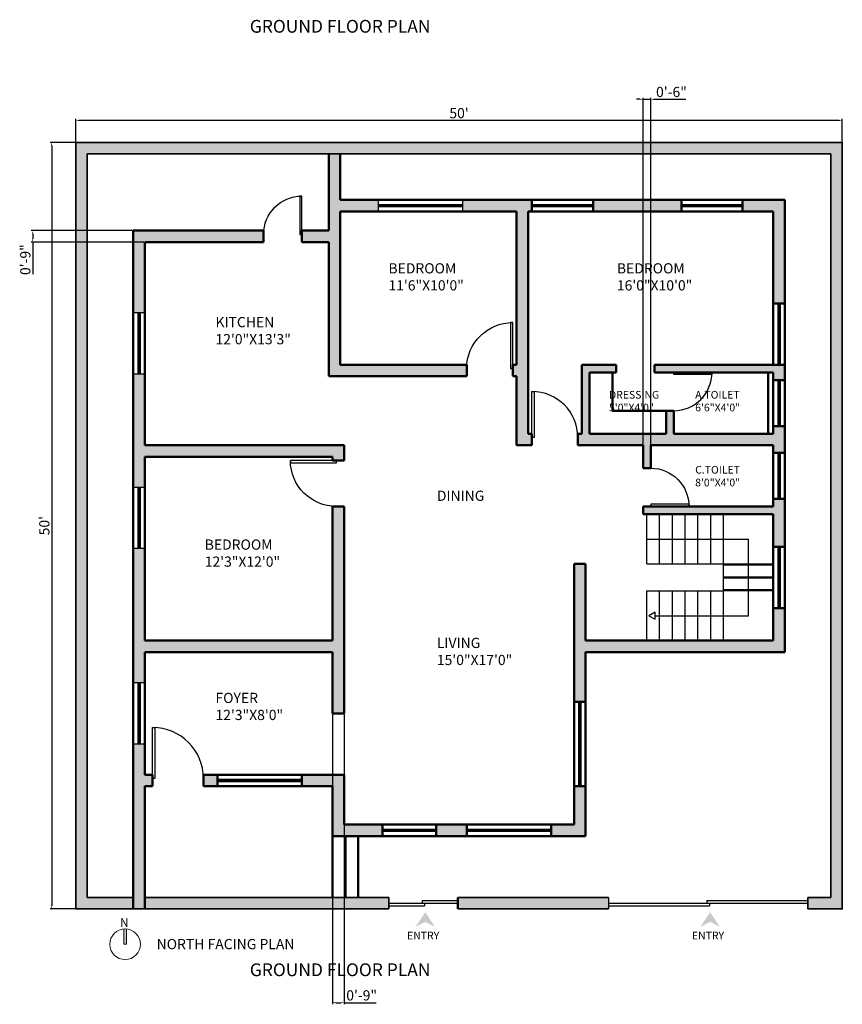
# Model space of a CAD drawing. Units: inches. Extents: x 2442 to 3851, y 589 to 2836.
# Tile 1 of 22: x 2450 to 3094, y 589 to 1359. Entities that reach past the tile are written whole.
import ezdxf

# ---------------------------------------------------------------- set-up
doc = ezdxf.new("R2010")
doc.units = ezdxf.units.IN
for name, color, linetype, lineweight in [('A-ANNO-DIMS', 2, 'Continuous', 18), ('A-ANNO-SYMB', 1, 'Continuous', 18), ('A-ANNO-TEXT', 7, 'Continuous', 18), ('A-AREA-IDEN', 7, 'Continuous', 18), ('A-DOOR', 4, 'Continuous', 25), ('A-FLOR-STRS', 3, 'Continuous', 25), ('A-GLAZ', 1, 'Continuous', 25), ('A-WALL', 7, 'Continuous', 50), ('A-WALL-PATT', 8, 'Continuous', 13), ('C-PROP', 7, 'Continuous', 35)]:
    doc.layers.add(name, color=color, linetype=linetype, lineweight=lineweight)
doc.styles.get("Standard").update_dxf_attribs({"font": 'arial.ttf'})
doc.dimstyles.new('ISO-25', dxfattribs={"dimtxt": 8, "dimasz": 2.5, "dimexe": 1.25, "dimexo": 0.625, "dimtad": 1, "dimlunit": 3, "dimtxsty": 'Standard', "dimcen": 2.5, "dimadec": 0, "dimazin": 0, "dimtfac": 1, "dimtmove": 0, "dimatfit": 3, "dimfxl": 1, "dimarcsym": 0})

# ---------------------------------------------------------------- blocks, each defined once
blk = doc.blocks.new('*U22')
for p, q in [((0, 0), (0, -6)), ((40, 0), (40, -6))]:
    blk.add_line(p, q)
blk.add_lwpolyline([(0, 0), (0, 40), (1.75, 40), (1.75, 0)], close=True)
blk.add_arc((0, 0), 40, 0, 90)
blk = doc.blocks.new('*U23')
for p, q in [((0, 0), (0, -6)), ((36, 0), (36, -6))]:
    blk.add_line(p, q)
blk.add_lwpolyline([(0, 0), (0, 36), (1.75, 36), (1.75, 0)], close=True)
blk.add_arc((0, 0), 36, 0, 90)
blk = doc.blocks.new('*U24')
for p, q in [((0, 0), (0, -6)), ((30, 0), (30, -6))]:
    blk.add_line(p, q)
blk.add_lwpolyline([(0, 0), (0, 30), (1.75, 30), (1.75, 0)], close=True)
blk.add_arc((0, 0), 30, 0, 90)
blk = doc.blocks.new('*D33')
at = {"layer": 'A-ANNO-DIMS', "color": 0, "lineweight": -2, "transparency": 16777216}
for p, q in [((2493.6, 1263.95), (2493.6, 1281.73)), ((3091.1, 1280.48), (2496.1, 1280.48)), ((3093.6, 1263.95), (3093.6, 1281.73))]:
    blk.add_line(p, q, dxfattribs=at)
at = {"layer": 'A-ANNO-DIMS', "color": 0, "transparency": 16777216}
for points in [[(2496.1, 1280.9), (2496.1, 1280.07), (2493.6, 1280.48)], [(3091.1, 1280.9), (3091.1, 1280.07), (3093.6, 1280.48)]]:
    blk.add_solid(points, dxfattribs=at)
at = {"layer": 'Defpoints', "color": 0, "transparency": 16777216}
for p in [(2493.6, 1280.48), (2493.6, 1263.32), (3093.6, 1263.32)]:
    blk.add_point(p, dxfattribs=at)
at = {"layer": 'A-ANNO-DIMS', "color": 0, "transparency": 16777216, "insert": (2793.6, 1285.19), "char_height": 8, "attachment_point": 5}
blk.add_mtext("50'", dxfattribs=at)
blk = doc.blocks.new('*D34')
at = {"layer": 'A-ANNO-DIMS', "color": 0, "lineweight": -2, "transparency": 16777216}
for p, q in [((2492.97, 1263.32), (2473.47, 1263.32)), ((2474.72, 1260.82), (2474.72, 665.82)), ((2492.97, 663.32), (2473.47, 663.32))]:
    blk.add_line(p, q, dxfattribs=at)
at = {"layer": 'A-ANNO-DIMS', "color": 0, "transparency": 16777216}
for points in [[(2474.3, 1260.82), (2475.14, 1260.82), (2474.72, 1263.32)], [(2474.3, 665.82), (2475.14, 665.82), (2474.72, 663.32)]]:
    blk.add_solid(points, dxfattribs=at)
at = {"layer": 'Defpoints', "color": 0, "transparency": 16777216}
for p in [(2493.6, 1263.32), (2474.72, 663.32), (2493.6, 663.32)]:
    blk.add_point(p, dxfattribs=at)
at = {"layer": 'A-ANNO-DIMS', "color": 0, "transparency": 16777216, "insert": (2470.01, 963.32), "char_height": 8, "attachment_point": 5, "rotation": 90}
blk.add_mtext("50'", dxfattribs=at)
blk = doc.blocks.new('NORTH-ARROW')
at = {"transparency": 33554687}
h = blk.add_hatch(color=256, dxfattribs=at)
h.dxf.hatch_style = 1
h.paths.add_polyline_path([(13, 12), (11, 12), (11, 23.96, -0.020861), (12, 24, -0.020861), (13, 23.96)])
for p, q in [((11, 24), (11, 12)), ((13, 12), (13, 23.96)), ((11, 12), (13, 12))]:
    blk.add_line(p, q)
blk.add_circle((12, 12), 12)
blk.add_text('N', height=6.9).set_placement((7.98, 25.6))
blk = doc.blocks.new('*D258')
at = {"layer": 'A-ANNO-DIMS', "color": 0, "lineweight": -2, "transparency": 16777216}
for p, q in [((2537.97, 1194.32), (2458.6, 1194.32)), ((2459.85, 1191.82), (2459.85, 1187.82)), ((2546.97, 1185.32), (2458.6, 1185.32)), ((2459.85, 1185.32), (2459.85, 1160.31))]:
    blk.add_line(p, q, dxfattribs=at)
at = {"layer": 'A-ANNO-DIMS', "color": 0, "transparency": 16777216}
for points in [[(2459.43, 1191.82), (2460.27, 1191.82), (2459.85, 1194.32)], [(2459.43, 1187.82), (2460.27, 1187.82), (2459.85, 1185.32)]]:
    blk.add_solid(points, dxfattribs=at)
at = {"layer": 'Defpoints', "color": 0, "transparency": 16777216}
for p in [(2538.6, 1194.32), (2459.85, 1185.32), (2547.6, 1185.32)]:
    blk.add_point(p, dxfattribs=at)
at = {"layer": 'A-ANNO-DIMS', "color": 0, "transparency": 16777216, "insert": (2455.14, 1171.56), "char_height": 8, "attachment_point": 5, "rotation": 90}
blk.add_mtext('0\'-9"', dxfattribs=at)
blk = doc.blocks.new('*D259')
at = {"layer": 'A-ANNO-DIMS', "color": 0, "lineweight": -2, "transparency": 16777216}
for p, q in [((2694.6, 815.7), (2694.6, 588.64)), ((2703.6, 815.7), (2703.6, 588.64)), ((2697.1, 589.89), (2701.1, 589.89)), ((2703.6, 589.89), (2728.61, 589.89))]:
    blk.add_line(p, q, dxfattribs=at)
at = {"layer": 'A-ANNO-DIMS', "color": 0, "transparency": 16777216}
for points in [[(2697.1, 590.31), (2697.1, 589.47), (2694.6, 589.89)], [(2701.1, 590.31), (2701.1, 589.47), (2703.6, 589.89)]]:
    blk.add_solid(points, dxfattribs=at)
at = {"layer": 'Defpoints', "color": 0, "transparency": 16777216}
for p in [(2694.6, 816.32), (2703.6, 816.32), (2703.6, 589.89)]:
    blk.add_point(p, dxfattribs=at)
at = {"layer": 'A-ANNO-DIMS', "color": 0, "transparency": 16777216, "insert": (2717.36, 594.6), "char_height": 8, "attachment_point": 5}
blk.add_mtext('0\'-9"', dxfattribs=at)
blk = doc.blocks.new('*D260')
at = {"layer": 'A-ANNO-DIMS', "color": 0, "lineweight": -2, "transparency": 16777216}
for p, q in [((2935.1, 1297.07), (2932.6, 1297.07)), ((2937.6, 1008.95), (2937.6, 1298.32)), ((2937.6, 1297.07), (2943.6, 1297.07)), ((2943.6, 1008.95), (2943.6, 1298.32)), ((2946.1, 1297.07), (2971.11, 1297.07))]:
    blk.add_line(p, q, dxfattribs=at)
at = {"layer": 'A-ANNO-DIMS', "color": 0, "transparency": 16777216}
for points in [[(2935.1, 1297.49), (2935.1, 1296.66), (2937.6, 1297.07)], [(2946.1, 1297.49), (2946.1, 1296.66), (2943.6, 1297.07)]]:
    blk.add_solid(points, dxfattribs=at)
at = {"layer": 'Defpoints', "color": 0, "transparency": 16777216}
for p in [(2943.6, 1297.07), (2937.6, 1008.32), (2943.6, 1008.32)]:
    blk.add_point(p, dxfattribs=at)
at = {"layer": 'A-ANNO-DIMS', "color": 0, "transparency": 16777216, "insert": (2959.86, 1301.78), "char_height": 8, "attachment_point": 5}
blk.add_mtext('0\'-6"', dxfattribs=at)

msp = doc.modelspace()

# ---------------------------------------------------------------- hatches: boundary and pattern name
at = {"layer": 'A-ANNO-SYMB'}
h = msp.add_hatch(color=256, dxfattribs=at)
h.dxf.hatch_style = 1
h.paths.add_polyline_path([(2767.136, 660.714), (2759.585, 649.389), (2767.136, 653.164), (2774.686, 649.389)])
h = msp.add_hatch(color=256, dxfattribs=at)
h.dxf.hatch_style = 1
h.paths.add_polyline_path([(2990.092, 660.714), (2982.542, 649.389), (2990.092, 653.164), (2997.642, 649.389)])
at = {"layer": 'A-WALL-PATT'}
h = msp.add_hatch(color=256, dxfattribs=at)
h.dxf.hatch_style = 1
h.paths.add_polyline_path([(2493.599, 663.323), (2538.599, 663.323), (2538.599, 672.323), (2502.599, 672.323), (2502.599, 1254.323), (3084.599, 1254.323), (3084.599, 672.323), (3066.599, 672.323), (3066.599, 663.323), (3093.599, 663.323), (3093.599, 1263.323), (2493.599, 1263.323)])
h.paths.add_polyline_path([(2910.599, 663.323), (2910.599, 664.323), (2910.599, 672.323), (2792.599, 672.323), (2792.599, 663.323)], flags=17)
h.paths.add_polyline_path([(2738.599, 663.323), (2738.599, 672.323), (2547.599, 672.323), (2547.599, 663.323)], flags=17)
h = msp.add_hatch(color=256, dxfattribs=at)
h.dxf.hatch_style = 1
h.paths.add_polyline_path([(2640.599, 1185.323), (2640.599, 1191.323), (2640.599, 1194.323), (2538.599, 1194.323), (2538.599, 1129.823), (2547.599, 1129.823), (2547.599, 1185.323)])
h.paths.add_polyline_path([(2700.599, 1209.323), (2730.599, 1209.323), (2730.599, 1218.323), (2700.599, 1218.323), (2700.599, 1254.323), (2691.599, 1254.323), (2691.599, 1194.323), (2670.599, 1194.323), (2670.599, 1191.323), (2670.599, 1185.323), (2691.599, 1185.323), (2691.599, 1080.323), (2799.599, 1080.323), (2799.599, 1086.323), (2799.599, 1089.323), (2700.599, 1089.323)])
h.paths.add_polyline_path([(2838.599, 1209.323), (2838.599, 1089.323), (2835.599, 1089.323), (2835.599, 1086.323), (2835.599, 1080.323), (2838.599, 1080.323), (2838.599, 1026.323), (2850.599, 1026.323), (2850.599, 1032.323), (2850.599, 1035.323), (2847.599, 1035.323), (2847.599, 1209.323), (2850.599, 1209.323), (2850.599, 1218.323), (2796.599, 1218.323), (2796.599, 1209.323)])
h.paths.add_polyline_path([(2898.599, 1218.323), (2898.599, 1209.323), (2967.599, 1209.323), (2967.599, 1218.323)])
h.paths.add_polyline_path([(3048.599, 1218.323), (3015.599, 1218.323), (3015.599, 1209.323), (3039.599, 1209.323), (3039.599, 1137.323), (3048.599, 1137.323)])
h.paths.add_polyline_path([(3039.599, 1083.323), (3039.599, 1077.323), (3048.599, 1077.323), (3048.599, 1089.323), (2946.599, 1089.323), (2946.599, 1083.323)])
h.paths.add_polyline_path([(2961.599, 1035.323), (2961.599, 1053.323), (2955.599, 1053.323), (2955.599, 1035.323), (2895.599, 1035.323), (2895.599, 1083.323), (2916.599, 1083.323), (2916.599, 1089.323), (2889.599, 1089.323), (2889.599, 1035.323), (2886.599, 1035.323), (2886.599, 1026.323), (2937.599, 1026.323), (2937.599, 1008.323), (2943.599, 1008.323), (2943.599, 1026.323), (3039.599, 1026.323), (3039.599, 1020.323), (3048.599, 1020.323), (3048.599, 1041.323), (3039.599, 1041.323), (3039.599, 1035.323)])
h.paths.add_polyline_path([(2538.599, 993.323), (2547.599, 993.323), (2547.599, 1017.323), (2694.599, 1017.323), (2694.599, 1014.323), (2697.599, 1014.323), (2703.599, 1014.323), (2703.599, 1026.323), (2547.599, 1026.323), (2547.599, 1081.823), (2538.599, 1081.823)])
h.paths.add_polyline_path([(2538.599, 840.323), (2547.599, 840.323), (2547.599, 864.323), (2694.599, 864.323), (2694.599, 816.323), (2703.599, 816.323), (2703.599, 978.323), (2697.599, 978.323), (2694.599, 978.323), (2694.599, 873.323), (2547.599, 873.323), (2547.599, 945.323), (2538.599, 945.323)])
h.paths.add_polyline_path([(2547.599, 759.323), (2553.599, 759.323), (2553.599, 765.323), (2553.599, 768.323), (2547.599, 768.323), (2547.599, 792.323), (2538.599, 792.323), (2538.599, 663.323), (2547.599, 663.323)])
h.paths.add_polyline_path([(2703.599, 768.323), (2670.599, 768.323), (2670.599, 759.323), (2694.599, 759.323), (2694.599, 720.323), (2733.599, 720.323), (2733.599, 729.323), (2703.599, 729.323)])
h.paths.add_polyline_path([(2593.599, 759.323), (2604.599, 759.323), (2604.599, 768.323), (2593.599, 768.323)])
h.paths.add_polyline_path([(2799.599, 720.323), (2799.599, 729.323), (2775.599, 729.323), (2775.599, 720.323)])
h.paths.add_polyline_path([(2892.599, 720.323), (2892.599, 759.323), (2883.599, 759.323), (2883.599, 729.323), (2865.599, 729.323), (2865.599, 720.323)])
h.paths.add_polyline_path([(2883.599, 825.323), (2892.599, 825.323), (2892.599, 864.323), (3048.599, 864.323), (3048.599, 898.823), (3039.599, 898.823), (3039.599, 873.323), (2892.599, 873.323), (2892.599, 933.323), (2883.599, 933.323)])
h.paths.add_polyline_path([(3039.599, 946.823), (3048.599, 946.823), (3048.599, 984.323), (3039.599, 984.323), (3039.599, 978.323), (2937.599, 978.323), (2937.599, 972.323), (3039.599, 972.323)])

# ---------------------------------------------------------------- linework, layer by layer
at = {"layer": 'A-FLOR-STRS'}
for p, q in [((2940.599, 933.323), (2940.599, 972.323)), ((2950.599, 933.323), (2950.599, 972.323)), ((2960.599, 933.323), (2960.599, 972.323)), ((2970.599, 933.323), (2970.599, 972.323)), ((2980.599, 933.323), (2980.599, 972.323)), ((2990.599, 933.323), (2990.599, 972.323)), ((3000.599, 912.323), (3000.599, 972.323)), ((2940.599, 952.823), (3020.099, 952.823)), ((3020.099, 892.823), (3020.099, 952.823)), ((2940.599, 933.323), (3000.599, 933.323)), ((2940.599, 912.323), (3000.599, 912.323)), ((2947.056, 892.823), (3020.099, 892.823))]:
    msp.add_line(p, q, dxfattribs=at)
at = {"layer": 'A-FLOR-STRS', "ltscale": 0.5}
for p, q in [((2940.599, 873.323), (2940.599, 912.323)), ((2950.599, 873.323), (2950.599, 912.323)), ((2960.599, 873.323), (2960.599, 912.323)), ((2970.599, 873.323), (2970.599, 912.323)), ((2980.599, 873.323), (2980.599, 912.323)), ((2990.599, 873.323), (2990.599, 912.323)), ((3000.599, 873.323), (3000.599, 912.323))]:
    msp.add_line(p, q, dxfattribs=at)
at = {"layer": 'A-FLOR-STRS'}
msp.add_lwpolyline([(2942.213, 892.823), (2947.056, 890.027), (2947.056, 895.619)], close=True, dxfattribs=at)
at = {"layer": 'A-GLAZ'}
for p, q in [((2730.599, 1209.323), (2730.599, 1218.323)), ((2796.599, 1209.323), (2796.599, 1218.323)), ((2547.599, 1129.823), (2538.599, 1129.823)), ((2547.599, 1081.823), (2538.599, 1081.823)), ((2547.599, 993.323), (2538.599, 993.323)), ((2547.599, 945.323), (2538.599, 945.323)), ((2547.599, 840.323), (2538.599, 840.323)), ((2547.599, 792.323), (2538.599, 792.323)), ((2910.599, 672.323), (2910.599, 663.323)), ((2738.599, 667.823), (2792.599, 667.823)), ((2738.599, 665.823), (2766.599, 665.823)), ((2764.599, 669.823), (2792.599, 669.823)), ((2764.599, 669.823), (2764.599, 667.823)), ((2766.599, 667.823), (2766.599, 665.823)), ((2910.599, 667.823), (3066.599, 667.823)), ((2910.599, 665.823), (2989.599, 665.823)), ((2910.599, 663.323), (2910.599, 664.323)), ((2987.599, 669.823), (3066.599, 669.823)), ((2987.599, 669.823), (2987.599, 667.823)), ((2989.599, 667.823), (2989.599, 665.823))]:
    msp.add_line(p, q, dxfattribs=at)
at = {"layer": 'A-WALL'}
for p, q in [((2691.599, 1194.323), (2691.599, 1254.323)), ((2700.599, 1218.323), (2700.599, 1254.323)), ((2700.599, 1218.323), (3048.599, 1218.323)), ((2850.599, 1209.323), (2850.599, 1218.323)), ((2898.599, 1209.323), (2898.599, 1218.323)), ((2967.599, 1209.323), (2967.599, 1218.323)), ((3015.599, 1209.323), (3015.599, 1218.323)), ((3048.599, 864.323), (3048.599, 1218.323)), ((2730.599, 1214.323), (2796.599, 1214.323)), ((2730.599, 1213.323), (2796.599, 1213.323)), ((2850.599, 1214.323), (2898.599, 1214.323)), ((2850.599, 1213.323), (2898.599, 1213.323)), ((2967.599, 1214.323), (3015.599, 1214.323)), ((2967.599, 1213.323), (3015.599, 1213.323)), ((2700.599, 1089.323), (2700.599, 1209.323)), ((2700.599, 1209.323), (2838.599, 1209.323)), ((2838.599, 1089.323), (2838.599, 1209.323)), ((2847.599, 1035.323), (2847.599, 1209.323)), ((2847.599, 1209.323), (3039.599, 1209.323)), ((3039.599, 1089.323), (3039.599, 1209.323)), ((2538.599, 1194.323), (2538.599, 663.323)), ((2538.599, 1194.323), (2640.599, 1194.323)), ((2640.599, 1185.323), (2640.599, 1194.323)), ((2670.599, 1185.323), (2670.599, 1194.323)), ((2670.599, 1194.323), (2691.599, 1194.323)), ((2547.599, 1185.323), (2547.599, 1026.323)), ((2547.599, 1185.323), (2640.599, 1185.323)), ((2670.599, 1185.323), (2691.599, 1185.323)), ((2691.599, 1080.323), (2691.599, 1185.323)), ((3039.599, 1137.323), (3048.599, 1137.323)), ((3043.599, 1089.323), (3043.599, 1137.323)), ((3044.599, 1089.323), (3044.599, 1137.323)), ((2542.599, 1129.823), (2542.599, 1081.823)), ((2543.599, 1129.823), (2543.599, 1081.823)), ((2700.599, 1089.323), (2799.599, 1089.323)), ((2799.599, 1080.323), (2799.599, 1089.323)), ((2835.599, 1080.323), (2835.599, 1089.323)), ((2835.599, 1089.323), (2838.599, 1089.323)), ((2889.599, 1035.323), (2889.599, 1089.323)), ((2889.599, 1089.323), (2916.599, 1089.323)), ((2916.599, 1083.323), (2916.599, 1089.323)), ((2946.599, 1083.323), (2946.599, 1089.323)), ((2946.599, 1089.323), (3048.599, 1089.323)), ((2691.599, 1080.323), (2799.599, 1080.323)), ((2835.599, 1080.323), (2838.599, 1080.323)), ((2838.599, 1026.323), (2838.599, 1080.323)), ((2895.599, 1035.323), (2895.599, 1083.323)), ((2895.599, 1083.323), (2916.599, 1083.323)), ((2913.599, 1053.323), (2913.599, 1083.323)), ((2946.599, 1083.323), (3039.599, 1083.323)), ((3035.599, 1035.323), (3035.599, 1083.323)), ((3039.599, 1035.323), (3039.599, 1083.323)), ((3039.599, 1077.323), (3048.599, 1077.323)), ((3043.599, 1041.323), (3043.599, 1077.323)), ((3044.599, 1041.323), (3044.599, 1077.323)), ((2913.599, 1053.323), (2955.599, 1053.323)), ((2955.599, 1035.323), (2955.599, 1053.323)), ((2955.599, 1053.323), (2961.599, 1053.323)), ((2961.599, 1035.323), (2961.599, 1053.323)), ((3039.599, 1041.323), (3048.599, 1041.323)), ((2847.599, 1035.323), (2850.599, 1035.323)), ((2850.599, 1026.323), (2850.599, 1035.323)), ((2886.599, 1026.323), (2886.599, 1035.323)), ((2886.599, 1035.323), (2889.599, 1035.323)), ((2895.599, 1035.323), (2955.599, 1035.323)), ((2961.599, 1035.323), (3039.599, 1035.323)), ((2547.599, 1026.323), (2703.599, 1026.323)), ((2703.599, 1014.323), (2703.599, 1026.323)), ((2838.599, 1026.323), (2850.599, 1026.323)), ((2886.599, 1026.323), (2937.599, 1026.323)), ((2937.599, 1008.323), (2937.599, 1026.323)), ((2943.599, 1008.323), (2943.599, 1026.323)), ((2943.599, 1026.323), (3039.599, 1026.323)), ((3039.599, 978.323), (3039.599, 1026.323)), ((3039.599, 1020.323), (3048.599, 1020.323)), ((3043.599, 984.323), (3043.599, 1020.323)), ((3044.599, 984.323), (3044.599, 1020.323)), ((2547.599, 1017.323), (2547.599, 873.323)), ((2547.599, 1017.323), (2694.599, 1017.323)), ((2694.599, 1014.323), (2694.599, 1017.323)), ((2694.599, 1014.323), (2703.599, 1014.323)), ((2937.599, 1008.323), (2943.599, 1008.323)), ((2542.599, 993.323), (2542.599, 945.323)), ((2543.599, 993.323), (2543.599, 945.323)), ((3039.599, 984.323), (3048.599, 984.323)), ((2694.599, 873.323), (2694.599, 978.323)), ((2694.599, 978.323), (2703.599, 978.323)), ((2703.599, 816.323), (2703.599, 978.323)), ((2937.599, 972.323), (2937.599, 978.323)), ((2937.599, 978.323), (3039.599, 978.323)), ((2937.599, 972.323), (3039.599, 972.323)), ((3039.599, 873.323), (3039.599, 972.323)), ((3039.599, 946.823), (3048.599, 946.823)), ((3043.599, 898.823), (3043.599, 946.823)), ((3044.599, 898.823), (3044.599, 946.823)), ((2883.599, 933.323), (2892.599, 933.323)), ((2883.599, 729.323), (2883.599, 933.323)), ((2892.599, 873.323), (2892.599, 933.323)), ((3000.599, 932.823), (3039.599, 932.823)), ((3000.599, 922.823), (3039.599, 922.823)), ((3000.599, 912.823), (3039.599, 912.823)), ((3039.599, 898.823), (3048.599, 898.823)), ((2547.599, 873.323), (2694.599, 873.323)), ((2892.599, 873.323), (3039.599, 873.323)), ((2547.599, 864.323), (2547.599, 768.323)), ((2547.599, 864.323), (2694.599, 864.323)), ((2694.599, 816.323), (2694.599, 864.323)), ((2892.599, 720.323), (2892.599, 864.323)), ((2892.599, 864.323), (3048.599, 864.323)), ((2542.599, 840.323), (2542.599, 792.323)), ((2543.599, 840.323), (2543.599, 792.323)), ((2883.599, 825.323), (2892.599, 825.323)), ((2887.599, 759.323), (2887.599, 825.323)), ((2888.599, 759.323), (2888.599, 825.323)), ((2694.599, 816.323), (2703.599, 816.323)), ((2547.599, 768.323), (2553.599, 768.323)), ((2553.599, 768.323), (2553.599, 759.323)), ((2593.599, 768.323), (2593.599, 759.323)), ((2593.599, 768.323), (2703.599, 768.323)), ((2604.599, 759.323), (2604.599, 768.323)), ((2604.599, 764.323), (2670.599, 764.323)), ((2604.599, 763.323), (2670.599, 763.323)), ((2670.599, 759.323), (2670.599, 768.323)), ((2703.599, 729.323), (2703.599, 768.323)), ((2547.599, 759.323), (2547.599, 663.323)), ((2547.599, 759.323), (2553.599, 759.323)), ((2593.599, 759.323), (2694.599, 759.323)), ((2694.599, 672.323), (2694.599, 759.323)), ((2883.599, 759.323), (2892.599, 759.323)), ((2703.599, 729.323), (2883.599, 729.323)), ((2733.599, 720.323), (2733.599, 729.323)), ((2733.599, 725.323), (2775.599, 725.323)), ((2775.599, 720.323), (2775.599, 729.323)), ((2799.599, 720.323), (2799.599, 729.323)), ((2799.599, 725.323), (2865.599, 725.323)), ((2865.599, 720.323), (2865.599, 729.323)), ((2694.599, 720.323), (2892.599, 720.323)), ((2704.599, 672.323), (2704.599, 720.323)), ((2714.599, 672.323), (2714.599, 720.323)), ((2733.599, 724.323), (2775.599, 724.323)), ((2799.599, 724.323), (2865.599, 724.323)), ((2792.599, 663.323), (2792.599, 672.323))]:
    msp.add_line(p, q, dxfattribs=at)
at = {"layer": 'C-PROP'}
for p, q in [((2738.599, 663.323), (2738.599, 672.323)), ((3066.599, 672.323), (3066.599, 663.323))]:
    msp.add_line(p, q, dxfattribs=at)
for points in [[(3066.599, 663.323), (3093.599, 663.323), (3093.599, 1263.323), (2493.599, 1263.323), (2493.599, 663.323), (2738.599, 663.323)], [(3066.599, 672.323), (3084.599, 672.323), (3084.599, 1254.323), (2502.599, 1254.323), (2502.599, 672.323), (2538.599, 672.323)], [(2547.599, 672.323), (2738.599, 672.323)], [(2792.599, 672.323), (2910.599, 672.323)], [(2792.599, 663.323), (2910.599, 663.323)]]:
    msp.add_lwpolyline(points, dxfattribs=at)

# ---------------------------------------------------------------- block references
at = {"layer": 'A-ANNO-SYMB'}
msp.add_blockref('NORTH-ARROW', (2520.188, 623.64), dxfattribs=at)
at = {"layer": 'A-DOOR', "xscale": -1}
for name, p in [('*U24', (2670.599, 1191.323)), ('*U23', (2835.599, 1086.323))]:
    msp.add_blockref(name, p, dxfattribs=at)
at = {"layer": 'A-DOOR', "rotation": 269.9999999999969}
msp.add_blockref('*U24', (2961.599, 1083.323), dxfattribs=at)
at = {"layer": 'A-DOOR'}
for name, p in [('*U23', (2850.599, 1032.323)), ('*U22', (2553.599, 765.323))]:
    msp.add_blockref(name, p, dxfattribs=at)
at = {"layer": 'A-DOOR', "xscale": -1}
for name, p, rotation in [('*U23', (2697.599, 1014.323), 90), ('*U24', (2943.599, 978.323), 270)]:
    msp.add_blockref(name, p, dxfattribs=dict(at, rotation=rotation))

# ---------------------------------------------------------------- texts
at = {"layer": 'A-ANNO-TEXT', "attachment_point": 1}
for s, insert, char_height in [('{\\fTimes New Roman|b0|i0|c0|p18;GROUND FLOOR PLAN}', (2629.794, 1359.217), 10), ('{\\fTimes New Roman|b0|i0|c0|p18;NORTH FACING PLAN}', (2556.881, 639.763), 8), ('{\\fTimes New Roman|b0|i0|c0|p18;ENTRY}', (2752.918, 645.482), 6), ('{\\fTimes New Roman|b0|i0|c0|p18;ENTRY}', (2975.874, 645.482), 6), ('{\\fTimes New Roman|b0|i0|c0|p18;GROUND FLOOR PLAN}', (2629.794, 620.676), 10)]:
    msp.add_mtext_dynamic_manual_height_columns(s, width=196.26071, gutter_width=12.5, heights=[0], dxfattribs=dict(at, insert=insert, char_height=char_height))
at = {"layer": 'A-AREA-IDEN', "attachment_point": 1}
for s, insert, char_height in [('{\\fTimes New Roman|b0|i0|c0|p18;BEDROOM\\P11\'6"X10\'0"}', (2738.331, 1168.758), 8), ('{\\fTimes New Roman|b0|i0|c0|p18;BEDROOM\\P16\'0"X10\'0"}', (2917.154, 1168.758), 8), ('{\\fTimes New Roman|b0|i0|c0|p18;KITCHEN\\P12\'0"X13\'3"}', (2602.937, 1126.619), 8), ('{\\fTimes New Roman|b0|i0|c0|p18;DRESSING\\P5\'0"X4\'0"}', (2910.952, 1068.783), 6), ('{\\fTimes New Roman|b0|i0|c0|p18;A.TOILET\\P6\'6"X4\'0"}', (2978.437, 1068.783), 6), ('{\\fTimes New Roman|b0|i0|c0|p18;C.TOILET\\P8\'0"X4\'0"}', (2978.437, 1010.077), 6), ('{\\fTimes New Roman|b0|i0|c0|p18;DINING}', (2776.221, 990.757), 8), ('{\\fTimes New Roman|b0|i0|c0|p18;BEDROOM\\P12\'3"X12\'0"}', (2594.523, 952.505), 8), ('{\\fTimes New Roman|b0|i0|c0|p18;LIVING\\P15\'0"X17\'0"}', (2776.221, 875.541), 8), ('{\\fTimes New Roman|b0|i0|c0|p18;FOYER\\P12\'3"X8\'0"}', (2602.937, 832.497), 8)]:
    msp.add_mtext_dynamic_manual_height_columns(s, width=110.76054, gutter_width=12.5, heights=[0], dxfattribs=dict(at, insert=insert, char_height=char_height))

# ---------------------------------------------------------------- dimensions: what is measured, and where the dimension line sits
at = {"layer": 'A-ANNO-DIMS'}
for base, p1, p2, override, picture, middle in [((2943.599, 1297.073), (2937.599, 1008.323), (2943.599, 1008.323), {"dimdec": 1, "dimlfac": 1, "dimrnd": 0, "dimzin": 1, "dimdsep": 46, "dimlunit": 4, "dimfrac": 2}, '*D260', (2959.857, 1301.782)), ((2493.599, 1280.482), (3093.599, 1263.323), (2493.599, 1263.323), {"dimclrd": 0, "dimclre": 0, "dimclrt": 0}, '*D33', (2793.599, 1285.191)), ((2703.599, 589.89), (2694.599, 816.323), (2703.599, 816.323), {"dimdec": 1, "dimlfac": 1, "dimrnd": 0, "dimzin": 1, "dimdsep": 46, "dimlunit": 4, "dimfrac": 2}, '*D259', (2717.357, 594.6))]:
    dim = msp.add_linear_dim(base=base, p1=p1, p2=p2, dimstyle='ISO-25', override=override, dxfattribs=at)
    dim.commit()
    dim.dimension.update_dxf_attribs({"geometry": picture, "text_midpoint": middle})
for base, p1, p2, override, picture, middle in [((2474.719, 663.323), (2493.599, 1263.323), (2493.599, 663.323), {"dimclrd": 0, "dimclre": 0, "dimclrt": 0}, '*D34', (2470.009, 963.323)), ((2459.849, 1185.323), (2538.599, 1194.323), (2547.599, 1185.323), {"dimdec": 1, "dimlfac": 1, "dimrnd": 0, "dimzin": 1, "dimdsep": 46, "dimlunit": 4, "dimfrac": 2}, '*D258', (2455.139, 1171.565))]:
    dim = msp.add_linear_dim(base=base, p1=p1, p2=p2, angle=90, dimstyle='ISO-25', override=override, dxfattribs=at)
    dim.commit()
    dim.dimension.update_dxf_attribs({"geometry": picture, "text_midpoint": middle})

doc.saveas('drawing.dxf')
